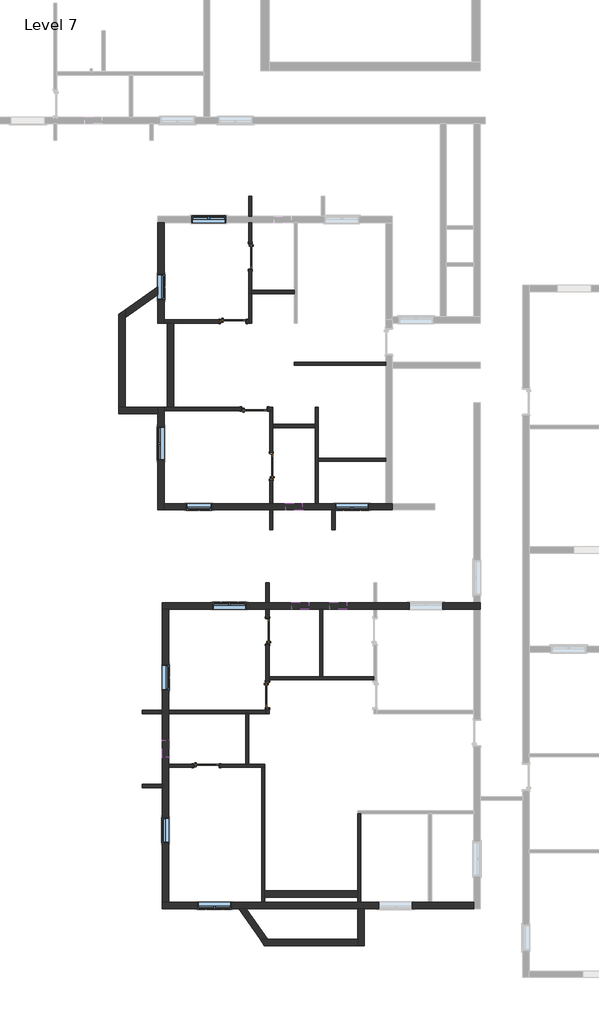
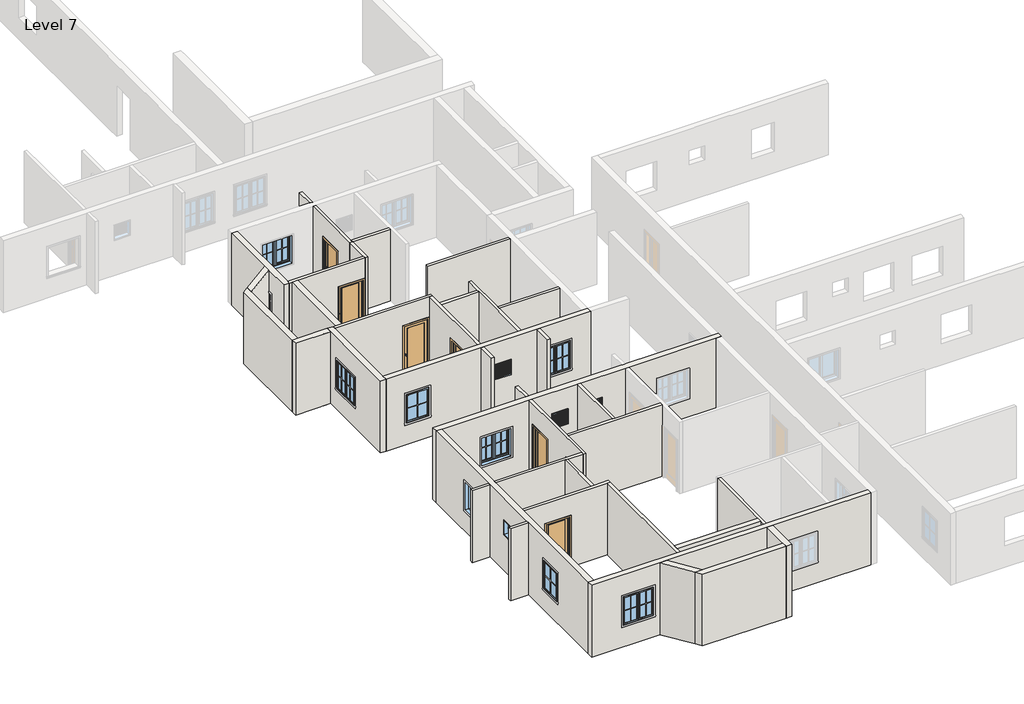
# One storey, part 1 of 7: 39 walls, 13 windows, 7 doors.
# Revit data of these elements (continued)
# Element 50 (IfcWindow, "Window-Awning-Single : 36\" x 48\"") (continued)
#   Interior Wall Closure = 0' - 2 1/4"
#   Frame Extension = 0' - 0 1/4"
#   Exterior Wall Closure = 0' - 1 1/4"
#   Interior Trim Visibility = yes
#   Exterior Trim Visibility = yes
#   Phase Created = New Construction
#   Materials on its faces: "Wood - Stained", "Glass", "Clad - White"
# Element 51 (IfcWindow, "Window-Casement-Double : 4' x 4'")
#   Mark = "184"
#   Window Inset = 0' - 0"
#   Interior Wall Closure = 0' - 2 1/4"
#   Frame Extension = 0' - 0 1/4"
#   Exterior Wall Closure = 0' - 1 1/4"
#   Interior Trim Visibility = yes
#   Exterior Trim Visibility = yes
#   Phase Created = New Construction
#   Materials on its faces: "Wood - Stained", "Glass", "Clad - White"
# Element 52 (IfcWindow, "Window-Casement-Double : 4' x 4'")
#   Mark = "186"
#   Window Inset = 0' - 0"
#   Interior Wall Closure = 0' - 2 1/4"
#   Frame Extension = 0' - 0 1/4"
#   Exterior Wall Closure = 0' - 1 1/4"
#   Interior Trim Visibility = yes
#   Exterior Trim Visibility = yes
#   Phase Created = New Construction
#   Materials on its faces: "Wood - Stained", "Glass", "Clad - White"
# Element 53 (IfcWindow, "Window-Casement-Double : 4' x 4'")
#   Mark = "188"
#   Window Inset = 0' - 0"
#   Interior Wall Closure = 0' - 2 1/4"
#   Frame Extension = 0' - 0 1/4"
#   Exterior Wall Closure = 0' - 1 1/4"
#   Interior Trim Visibility = yes
#   Exterior Trim Visibility = yes
#   Phase Created = New Construction
#   Materials on its faces: "Wood - Stained", "Glass", "Clad - White"
# Element 54 (IfcWindow, "Window-Casement-Double : 4' x 4'")
#   Mark = "189"
#   Window Inset = 0' - 0"
#   Interior Wall Closure = 0' - 2 1/4"
#   Frame Extension = 0' - 0 1/4"
#   Exterior Wall Closure = 0' - 1 1/4"
#   Interior Trim Visibility = yes
#   Exterior Trim Visibility = yes
#   Phase Created = New Construction
#   Materials on its faces: "Wood - Stained", "Glass", "Clad - White"
# Element 55 (IfcWindow, "Window-Casement-Double : 4' x 4'")
#   Mark = "191"
#   Window Inset = 0' - 0"
#   Interior Wall Closure = 0' - 2 1/4"
#   Frame Extension = 0' - 0 1/4"
#   Exterior Wall Closure = 0' - 1 1/4"
#   Interior Trim Visibility = yes
#   Exterior Trim Visibility = yes
#   Phase Created = New Construction
#   Materials on its faces: "Wood - Stained", "Glass", "Clad - White"
# Element 56 (IfcWindow, "Window-Louvers : 24\" x 24\"")
#   Mark = "140"
#   Blade Width = 1' - 10 1/2"
#   Phase Created = New Construction
#   Materials on its faces: "Birch"
# Element 57 (IfcWindow, "Window-Louvers : 24\" x 24\"")
#   Mark = "143"
#   Blade Width = 1' - 10 1/2"
#   Phase Created = New Construction
#   Materials on its faces: "Birch"
# Element 58 (IfcWindow, "Window-Louvers : 24\" x 24\"")
#   Mark = "144"
#   Blade Width = 1' - 10 1/2"
#   Phase Created = New Construction
#   Materials on its faces: "Birch"
# Element 59 (IfcWindow, "Window-Louvers : 24\" x 24\"")
#   Mark = "146"
#   Blade Width = 1' - 10 1/2"
#   Phase Created = New Construction
#   Materials on its faces: "Birch"
# Materials
#   "Cherry": class "Wood", colour RGB 226 177 128, transparency 0, Description = "Prunus Serotina", Cost = 0
#   "Aluminum": class "Metal", colour RGB 247 247 247, transparency 0, Description = "Aluminum 6061", Cost = 0
#   "Wood - Stained": class "Wood", colour RGB 224 178 126, transparency 0, Cost = 0
#   "Glass": class "Glass", colour RGB 0 128 192, transparency 0.75, Description = "Soda Lime Glass", Cost = 0
#   "Clad - White": class "Wood", colour RGB 242 242 238, transparency 0, Cost = 0
#   "Birch": class "Wood", colour RGB 224 178 126, transparency 0, Description = "Betula Alleghaniensis", Cost = 0
#   "Default Wall": colour RGB 128 128 128, transparency 0, Cost = 0
